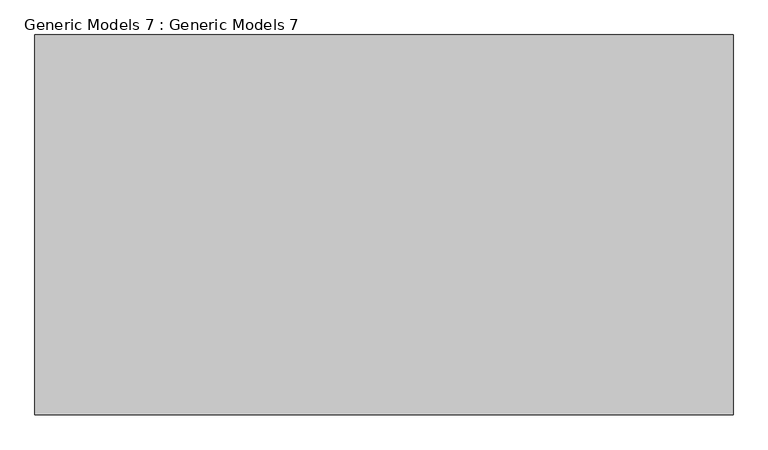
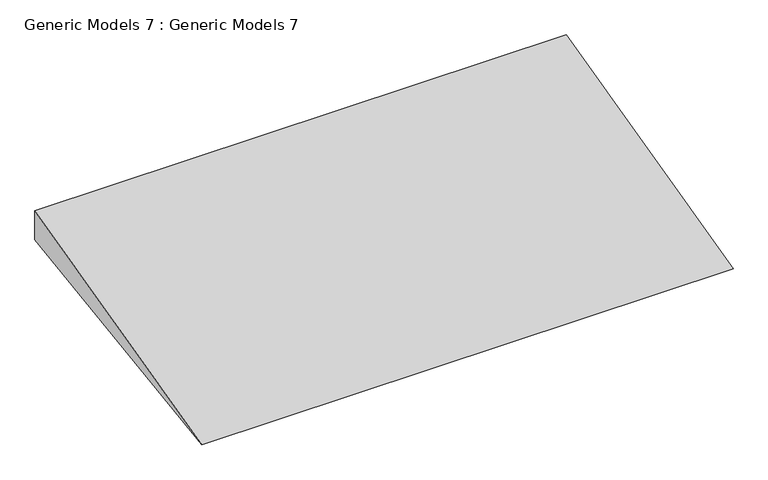
"""IFC4 building model written with IfcOpenShell, lengths in millimetres: proxy geometry, Generic Models 7 : Generic Models 7."""

from ifc_helpers import new_model, si_unit, frame, origin, place, context, project, spatial, polyline, outline, extrude, source, transform, mapped, element, save


def generic_models_7_generic_models_7_fbfc4c3c(model_context):
    return source(origin(), model_context, "Body", "SweptSolid", [
        extrude(outline(polyline([(-9891.3653461, -362.5441527), (-8437.2801707, 0.0), (-8437.2801707, -152.484342), (-9891.3653461, -362.5441527)])), frame((-2573.939433, 0.0, 0.0), z_axis=(1.0, 0.0, 0.0), x_axis=(0.0, 1.0, 0.0)), (0.0, 0.0, 1.0), 2672.6694491),
    ])


if __name__ == "__main__":
    model = new_model("IFC4")
    model_context = context("Model", 3, world=origin())
    ifc_project = project(units=[si_unit("LENGTHUNIT", "METRE", prefix="MILLI")], contexts=[model_context])
    site = spatial("IfcSite", under=ifc_project)
    building = spatial("IfcBuilding", under=site)
    placement = place(None, origin())
    generic_models_7_generic_models_7_shape = generic_models_7_generic_models_7_fbfc4c3c(model_context)
    element("IfcBuildingElementProxy", 1, Name="Generic Models 7 : Generic Models 7", ObjectType="Generic Models 7 : Generic Models 7", at=placement, inside=building, context=model_context, shape_type="MappedRepresentation", body=[
        mapped(generic_models_7_generic_models_7_shape, transform((0.0, 0.0, 0.0), x_axis=(1.0, 0.0, 0.0), y_axis=(0.0, 1.0, 0.0), z_axis=(0.0, 0.0, 1.0))),
    ])
    save(model, "model.ifc")
